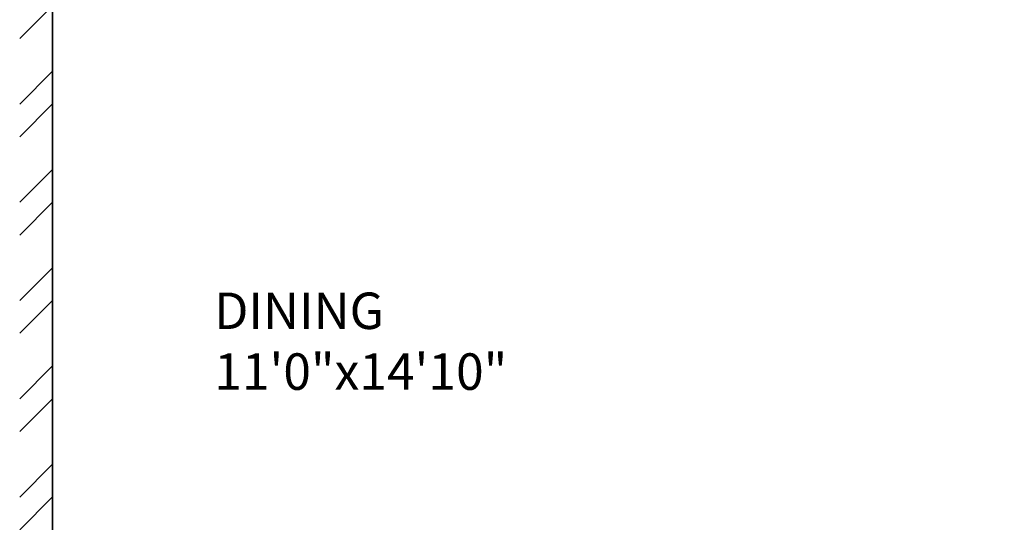
# Model space of a CAD drawing. Units: inches. Extents: x 1962 to 2771, y 1245 to 2660.
# Tile 12 of 114: x 2371 to 2506, y 1762 to 1831. Entities that reach past the tile are written whole.
import ezdxf

# ---------------------------------------------------------------- set-up
doc = ezdxf.new("R2010")
doc.units = ezdxf.units.IN
for name, color, linetype, lineweight in [('A-AREA-IDEN', 7, 'Continuous', 18), ('A-WALL', 7, 'Continuous', 35), ('A-WALL-PATT', 252, 'Continuous', 13)]:
    doc.layers.add(name, color=color, linetype=linetype, lineweight=lineweight)
doc.styles.get("Standard").update_dxf_attribs({"font": 'arial.ttf'})

msp = doc.modelspace()

# ---------------------------------------------------------------- hatches: boundary and pattern name
at = {"layer": 'A-WALL-PATT'}
h = msp.add_hatch(dxfattribs=at)
h.set_pattern_fill('ANSI32', color=256)
h.paths.add_polyline_path([(2090.8074, 2467.3437), (2141.6481, 2467.3437), (2141.6481, 2469.5937), (2141.6481, 2471.8437), (2086.3074, 2471.8437), (2086.3074, 2422.5333), (2090.8074, 2422.5333)])
h.paths.add_polyline_path([(2282.7664, 2471.8437), (2204.8982, 2471.8437), (2204.8982, 2467.3437), (2234.8074, 2467.3437), (2234.8074, 2311.3437), (2228.7492, 2311.3437), (2228.7492, 2306.8437), (2234.8074, 2306.8437), (2331.9227, 2306.8437), (2331.9227, 2309.0937), (2331.9227, 2311.3437), (2239.3074, 2311.3437), (2239.3074, 2467.3437), (2282.7664, 2467.3437), (2282.7664, 2469.5937)])
h.paths.add_polyline_path([(2471.4531, 2519.8437), (2552.011, 2519.8437), (2564.3996, 2519.8437), (2564.3996, 2511.1389), (2568.8996, 2511.1389), (2568.8996, 2524.3437), (2466.9531, 2524.3437), (2466.9531, 2471.8437), (2450.0749, 2471.8437), (2446.4672, 2471.8437), (2446.4672, 2467.3437), (2450.0749, 2467.3437), (2475.9988, 2467.3437), (2475.9988, 2469.5937), (2475.9988, 2471.8437), (2471.4531, 2471.8437)])
h.paths.add_polyline_path([(2575.2231, 2469.5937), (2575.2231, 2471.8437), (2568.8996, 2471.8437), (2568.8996, 2487.1389), (2564.3996, 2487.1389), (2564.3996, 2471.8437), (2556.511, 2471.8437), (2499.2904, 2471.8437), (2499.2904, 2467.3437), (2507.8074, 2467.3437), (2507.8074, 2311.3437), (2414.863, 2311.3437), (2414.863, 2306.8437), (2512.3074, 2306.8437), (2517.0114, 2306.8437), (2517.0114, 2309.0937), (2517.0114, 2311.3437), (2512.3074, 2311.3437), (2512.3074, 2467.3437), (2575.2231, 2467.3437)])
h.paths.add_polyline_path([(2660.8074, 2471.8437), (2600.9602, 2471.8437), (2600.9602, 2467.3437), (2656.3074, 2467.3437), (2656.3074, 2432.5704), (2660.8074, 2432.5704)])
h.paths.add_polyline_path([(2660.8074, 2372.5704), (2656.3074, 2372.5704), (2656.3074, 2311.3437), (2600.276, 2311.3437), (2600.276, 2309.0937), (2600.276, 2306.8437), (2656.3074, 2306.8437), (2656.3074, 2296.2593), (2660.8074, 2296.2593)])
h.paths.add_polyline_path([(2572.3074, 2306.8437), (2577.1385, 2306.8437), (2577.1385, 2311.3437), (2551.082, 2311.3437), (2551.082, 2306.8437), (2567.8074, 2306.8437), (2567.8074, 2258.8437), (2540.0574, 2258.8437), (2540.0574, 2256.5937), (2540.0574, 2254.3437), (2567.8074, 2254.3437), (2656.3074, 2254.3437), (2656.3074, 2236.9085), (2660.8074, 2236.9085), (2660.8074, 2272.2593), (2656.3074, 2272.2593), (2656.3074, 2258.8437), (2572.3074, 2258.8437)])
h.paths.add_polyline_path([(2512.3074, 2254.3437), (2518.8716, 2254.3437), (2518.8716, 2256.5937), (2518.8716, 2258.8437), (2507.8074, 2258.8437), (2507.8074, 2177.8437), (2567.8074, 2177.8437), (2567.8074, 2172.9628), (2572.3074, 2172.9628), (2572.3074, 2177.8437), (2656.3074, 2177.8437), (2656.3074, 2166.4846), (2660.8074, 2166.4846), (2660.8074, 2200.9085), (2656.3074, 2200.9085), (2656.3074, 2182.3437), (2512.3074, 2182.3437)])
h.paths.add_polyline_path([(2656.3074, 2129.8437), (2572.3074, 2129.8437), (2572.3074, 2150.3044), (2570.0574, 2150.3044), (2567.8074, 2150.3044), (2567.8074, 2129.8437), (2507.8074, 2129.8437), (2507.8074, 2116.3027), (2510.0574, 2116.3027), (2512.3074, 2116.3027), (2512.3074, 2125.3437), (2567.8074, 2125.3437), (2572.3074, 2125.3437), (2656.3074, 2125.3437)])
h.paths.add_polyline_path([(2090.8074, 2362.5333), (2086.3074, 2362.5333), (2086.3074, 2298.6242), (2090.8074, 2298.6242), (2090.8074, 2306.8437), (2174.8074, 2306.8437), (2174.8074, 2286.4178), (2179.3074, 2286.4178), (2179.3074, 2306.8437), (2192.8641, 2306.8437), (2192.8641, 2309.0937), (2192.8641, 2311.3437), (2090.8074, 2311.3437)])
h.paths.add_polyline_path([(2209.156, 2258.8437), (2179.3074, 2258.8437), (2179.3074, 2263.2236), (2177.0574, 2263.2236), (2174.8074, 2263.2236), (2174.8074, 2258.8437), (2090.8074, 2258.8437), (2090.8074, 2274.6242), (2086.3074, 2274.6242), (2086.3074, 2238.2967), (2088.5574, 2238.2967), (2090.8074, 2238.2967), (2090.8074, 2254.3437), (2209.156, 2254.3437)])
h.paths.add_polyline_path([(2090.8074, 2177.8437), (2234.8074, 2177.8437), (2234.8074, 2173.1428), (2239.3074, 2173.1428), (2239.3074, 2258.8437), (2230.8442, 2258.8437), (2230.8442, 2256.5937), (2230.8442, 2254.3437), (2234.8074, 2254.3437), (2234.8074, 2182.3437), (2090.8074, 2182.3437), (2090.8074, 2202.2967), (2086.3074, 2202.2967), (2086.3074, 2140.0389), (2090.8074, 2140.0389)])
h.paths.add_polyline_path([(2090.8074, 2080.0389), (2086.3074, 2080.0389), (2086.3074, 2033.8437), (2090.8074, 2033.8437)], flags=17)
h.paths.add_polyline_path([(2244.9405, 2033.8437), (2239.3074, 2033.8437), (2239.3074, 2142.0665), (2237.2592, 2142.0665), (2234.8074, 2142.0665), (2234.8074, 2033.8437), (2090.8074, 2033.8437), (2076.5204, 2033.8437), (2072.0204, 2033.8437), (2072.0204, 2000.4493), (2076.5204, 2000.4493), (2076.5204, 2029.3437), (2090.8074, 2029.3437), (2244.9405, 2029.3437), (2244.9405, 2031.5937)])
h.paths.add_polyline_path([(2234.8074, 1933.3437), (2076.5204, 1933.3437), (2076.5204, 1952.4493), (2074.2704, 1952.4493), (2072.0204, 1952.4493), (2072.0204, 1933.3437), (2072.0204, 1928.8437), (2234.8074, 1928.8437)])
h.paths.add_polyline_path([(2090.8074, 1928.8437), (2086.3074, 1928.8437), (2086.3074, 1906.5013), (2090.8074, 1906.5013)])
h.paths.add_polyline_path([(2090.8074, 1846.5013), (2086.3074, 1846.5013), (2086.3074, 1769.9917), (2088.5574, 1769.9917), (2090.8074, 1769.9917), (2090.8074, 1780.3437), (2234.8074, 1780.3437), (2234.8074, 1708.3437), (2230.3764, 1708.3437), (2230.3764, 1703.8437), (2239.3074, 1703.8437), (2239.3074, 1792.6669), (2237.0574, 1792.6669), (2234.8074, 1792.6669), (2234.8074, 1784.8437), (2090.8074, 1784.8437)])
h.paths.add_polyline_path([(2239.3074, 1928.8437), (2244.9405, 1928.8437), (2244.9405, 1931.0937), (2244.9405, 1933.3437), (2234.8074, 1933.3437), (2234.8074, 1928.8437), (2234.8074, 1825.5949), (2239.3074, 1825.5949)])
h.paths.add_polyline_path([(2148.0425, 1649.0937), (2148.0425, 1651.3437), (2090.8074, 1651.3437), (2090.8074, 1646.8437), (2148.0425, 1646.8437)], flags=0)
h.paths.add_polyline_path([(2207.5601, 1708.3437), (2090.8074, 1708.3437), (2090.8074, 1703.8437), (2174.8074, 1703.8437), (2174.8074, 1651.3437), (2170.4457, 1651.3437), (2170.4457, 1646.8437), (2195.9924, 1646.8437), (2195.9924, 1649.0937), (2195.9924, 1651.3437), (2179.3074, 1651.3437), (2179.3074, 1703.8437), (2207.5601, 1703.8437), (2207.5601, 1706.0937)])
h.paths.add_polyline_path([(2090.8074, 1733.9917), (2086.3074, 1733.9917), (2086.3074, 1696.1032), (2088.5574, 1696.1032), (2090.8074, 1696.1032)])
h.paths.add_polyline_path([(2090.8074, 1672.1032), (2086.3074, 1672.1032), (2086.3074, 1600.3335), (2090.8074, 1600.3335)])
h.paths.add_polyline_path([(2090.8074, 1540.3335), (2086.3074, 1540.3335), (2086.3074, 1486.3437), (2139.6766, 1486.3437), (2139.6766, 1490.8437), (2090.8074, 1490.8437)])
h.paths.add_polyline_path([(2302.3876, 1490.8437), (2239.3074, 1490.8437), (2239.3074, 1646.8437), (2335.9994, 1646.8437), (2335.9994, 1651.3437), (2229.884, 1651.3437), (2229.884, 1646.8437), (2234.8074, 1646.8437), (2234.8074, 1490.8437), (2202.7103, 1490.8437), (2202.7103, 1488.5937), (2202.7103, 1486.3437), (2275.0699, 1486.3437), (2275.0699, 1475.772), (2279.5699, 1475.772), (2279.5699, 1486.3437), (2302.3876, 1486.3437)])
h.paths.add_polyline_path([(2279.5699, 1451.772), (2275.0699, 1451.772), (2275.0699, 1438.3437), (2174.8074, 1438.3437), (2174.8074, 1486.3437), (2179.7922, 1486.3437), (2179.7922, 1490.8437), (2163.3585, 1490.8437), (2163.3585, 1488.5937), (2163.3585, 1486.3437), (2170.3074, 1486.3437), (2170.3074, 1433.8437), (2279.5699, 1433.8437)])
h.paths.add_polyline_path([(2427.2363, 1490.8437), (2375.8074, 1490.8437), (2375.8074, 1646.8437), (2381.6401, 1646.8437), (2381.6401, 1651.3437), (2365.887, 1651.3437), (2365.887, 1649.0937), (2365.887, 1646.8437), (2371.3074, 1646.8437), (2371.3074, 1490.8437), (2327.5627, 1490.8437), (2327.5627, 1488.5937), (2327.5627, 1486.3437), (2371.3074, 1486.3437), (2371.3074, 1433.8437), (2375.8074, 1433.8437), (2375.8074, 1486.3437), (2427.2363, 1486.3437)])
h.paths.add_polyline_path([(2512.3074, 1646.8437), (2519.4351, 1646.8437), (2519.4351, 1649.0937), (2519.4351, 1651.3437), (2507.8074, 1651.3437), (2416.0063, 1651.3437), (2416.0063, 1649.0937), (2416.0063, 1646.8437), (2507.8074, 1646.8437), (2507.8074, 1490.8437), (2497.0532, 1490.8437), (2497.0532, 1488.5937), (2497.0532, 1486.3437), (2574.9344, 1486.3437), (2574.9344, 1476.0181), (2579.4344, 1476.0181), (2579.4344, 1486.3437), (2584.4872, 1486.3437), (2584.3074, 1490.8437), (2512.3074, 1490.8437)])
h.paths.add_polyline_path([(2470.5091, 1486.3437), (2473.9767, 1486.3437), (2473.9767, 1490.8437), (2449.6605, 1490.8437), (2449.6605, 1488.5937), (2449.6605, 1486.3437), (2466.0091, 1486.3437), (2466.0091, 1433.8437), (2470.5091, 1433.8437), (2579.4344, 1433.8437), (2579.4344, 1452.0181), (2574.9344, 1452.0181), (2574.9344, 1438.3437), (2554.5091, 1438.3437), (2470.5091, 1438.3437)])
h.paths.add_polyline_path([(2656.3074, 1490.8437), (2611.86, 1490.8437), (2611.86, 1486.3437), (2656.3074, 1486.3437)])
h.paths.add_polyline_path([(2660.8074, 1532.7007), (2658.5574, 1532.7007), (2656.3074, 1532.7007), (2656.3074, 1486.3437), (2660.8074, 1486.3437)])
h.paths.add_polyline_path([(2660.8074, 1664.9663), (2656.3074, 1664.9663), (2656.3074, 1651.3437), (2602.2313, 1651.3437), (2602.2313, 1646.8437), (2656.3074, 1646.8437), (2656.3074, 1592.7007), (2660.8074, 1592.7007)])
h.paths.add_polyline_path([(2660.8074, 1724.5221), (2656.3074, 1724.5221), (2656.3074, 1703.8437), (2542.4725, 1703.8437), (2542.4725, 1699.3437), (2567.8074, 1699.3437), (2567.8074, 1651.3437), (2552.7766, 1651.3437), (2552.7766, 1649.0937), (2552.7766, 1646.8437), (2577.2878, 1646.8437), (2577.2878, 1649.0937), (2577.2878, 1651.3437), (2572.3074, 1651.3437), (2572.3074, 1699.3437), (2656.3074, 1699.3437), (2656.3074, 1688.9663), (2660.8074, 1688.9663)])
h.paths.add_polyline_path([(2660.8074, 1880.6524), (2656.3074, 1880.6524), (2656.3074, 1832.8437), (2512.3074, 1832.8437), (2512.3074, 1837.8959), (2507.8074, 1837.8959), (2507.8074, 1828.3437), (2567.8074, 1828.3437), (2567.8074, 1804.3437), (2572.3074, 1804.3437), (2572.3074, 1828.3437), (2656.3074, 1828.3437), (2656.3074, 1818.6778), (2660.8074, 1818.6778)])
h.paths.add_polyline_path([(2660.8074, 1794.6778), (2656.3074, 1794.6778), (2656.3074, 1780.3437), (2572.3074, 1780.3437), (2572.3074, 1783.0303), (2570.0574, 1783.0303), (2567.8074, 1783.0303), (2567.8074, 1780.3437), (2507.8074, 1780.3437), (2507.8074, 1699.3437), (2517.8858, 1699.3437), (2517.8858, 1701.5937), (2517.8858, 1703.8437), (2512.3074, 1703.8437), (2512.3074, 1775.8437), (2656.3074, 1775.8437), (2656.3074, 1760.5221), (2660.8074, 1760.5221)])
h.paths.add_polyline_path([(2660.8074, 1981.3437), (2660.8074, 2020.2808), (2658.5574, 2020.2808), (2656.3074, 2020.2808), (2656.3074, 1981.3437), (2512.3074, 1981.3437), (2512.3074, 2086.6996), (2507.8074, 2086.6996), (2507.8074, 1981.3437), (2375.8074, 1981.3437), (2375.8074, 1986.8505), (2373.5574, 1986.8505), (2371.3074, 1986.8505), (2371.3074, 1973.2607), (2375.8074, 1973.2607), (2375.8074, 1976.8437), (2507.8074, 1976.8437), (2507.8074, 1865.4281), (2510.0574, 1865.4281), (2512.3074, 1865.4281), (2512.3074, 1976.8437), (2660.8074, 1976.8437)])
h.paths.add_polyline_path([(2375.8074, 1940.297), (2373.5574, 1940.297), (2371.3074, 1940.297), (2371.3074, 1933.3437), (2278.4434, 1933.3437), (2278.4434, 1928.8437), (2371.3074, 1928.8437), (2371.3074, 1651.3437), (2375.8074, 1651.3437)])
h.paths.add_polyline_path([(2660.8074, 1976.8437), (2656.3074, 1976.8437), (2656.3074, 1940.6524), (2660.8074, 1940.6524)], flags=17)
h.paths.add_polyline_path([(2660.8074, 2142.4846), (2656.3074, 2142.4846), (2656.3074, 2080.2808), (2660.8074, 2080.2808)])
h.paths.add_polyline_path([(2381.4189, 2311.3437), (2375.8074, 2311.3437), (2375.8074, 2467.3437), (2424.7242, 2467.3437), (2424.7242, 2469.5937), (2424.7242, 2471.8437), (2375.8074, 2471.8437), (2375.8074, 2524.3437), (2371.3074, 2524.3437), (2371.3074, 2471.8437), (2307.2097, 2471.8437), (2307.2097, 2467.3437), (2371.3074, 2467.3437), (2371.3074, 2311.3437), (2366.8901, 2311.3437), (2366.8901, 2306.8437), (2371.3074, 2306.8437), (2371.3074, 2033.8437), (2279.6589, 2033.8437), (2279.6589, 2029.3437), (2371.3074, 2029.3437), (2371.3074, 2014.2598), (2375.8074, 2014.2598), (2375.8074, 2306.8437), (2381.4189, 2306.8437)])
h.paths.add_polyline_path([(2263.3074, 2524.3437), (2170.3074, 2524.3437), (2170.3074, 2519.8437), (2170.3074, 2471.8437), (2165.0312, 2471.8437), (2165.0312, 2467.3437), (2179.6721, 2467.3437), (2179.6721, 2469.5161), (2179.6721, 2471.8437), (2174.8074, 2471.8437), (2174.8074, 2519.8437), (2258.8074, 2519.8437), (2258.8074, 2511.6436), (2263.3074, 2511.6436)])
h.paths.add_polyline_path([(2245.0232, 1361.4123), (2492.9468, 1361.4123), (2492.9468, 1398.505), (2245.0232, 1398.505)], flags=9)
h.paths.add_polyline_path([(2388.1434, 2086.6936), (2425.0704, 2086.6936), (2425.0704, 2105.3509), (2388.1434, 2105.3509)], flags=9)
h.paths.add_polyline_path([(2404.922, 2242.6744), (2445.7337, 2242.6744), (2445.7337, 2261.3318), (2404.922, 2261.3318)], flags=9)
h.paths.add_polyline_path([(2269.4107, 2156.7935), (2306.3378, 2156.7935), (2306.3378, 2175.4508), (2269.4107, 2175.4508)], flags=9)
h.paths.add_polyline_path([(2269.3277, 2233.4343), (2306.2547, 2233.4343), (2306.2547, 2252.0917), (2269.3277, 2252.0917)], flags=9)
h.paths.add_polyline_path([(2431.6052, 2320.6922), (2470.4456, 2320.6922), (2470.4456, 2339.3495), (2431.6052, 2339.3495)], flags=25)
h.paths.add_polyline_path([(2249.6902, 2315.7608), (2288.5306, 2315.7608), (2288.5306, 2334.4182), (2249.6902, 2334.4182)], flags=25)
h.paths.add_polyline_path([(2096.9301, 2314.3181), (2135.7704, 2314.3181), (2135.7704, 2332.9755), (2096.9301, 2332.9755)], flags=25)
h.paths.add_polyline_path([(2134.3475, 2285.7089), (2161.4655, 2285.7089), (2161.4655, 2304.3662), (2134.3475, 2304.3662)], flags=9)
h.paths.add_polyline_path([(2126.5155, 2209.4076), (2159.9227, 2209.4076), (2159.9227, 2228.065), (2126.5155, 2228.065)], flags=25)
h.paths.add_polyline_path([(2110.5753, 2141.5299), (2149.4157, 2141.5299), (2149.4157, 2160.1872), (2110.5753, 2160.1872)], flags=25)
h.paths.add_polyline_path([(2249.8618, 1968.3317), (2286.3966, 1968.3317), (2286.3966, 1986.989), (2249.8618, 1986.989)], flags=9)
h.paths.add_polyline_path([(2395.9507, 1777.0051), (2436.7624, 1777.0051), (2436.7624, 1795.6625), (2395.9507, 1795.6625)], flags=9)
h.paths.add_polyline_path([(2398.5259, 1888.5651), (2435.0062, 1888.5651), (2435.0062, 1907.2224), (2398.5259, 1907.2224)], flags=25)
h.paths.add_polyline_path([(2259.3506, 1728.3559), (2296.2776, 1728.3559), (2296.2776, 1747.0132), (2259.3506, 1747.0132)], flags=9)
h.paths.add_polyline_path([(2271.3698, 1845.268), (2308.2968, 1845.268), (2308.2968, 1863.9253), (2271.3698, 1863.9253)], flags=9)
h.paths.add_polyline_path([(2120.9355, 1786.3027), (2159.7759, 1786.3027), (2159.7759, 1804.9601), (2120.9355, 1804.9601)], flags=25)
h.paths.add_polyline_path([(2121.3164, 1732.1043), (2154.7236, 1732.1043), (2154.7236, 1750.7616), (2121.3164, 1750.7616)], flags=25)
h.paths.add_polyline_path([(2118.3706, 1678.8997), (2147.5282, 1678.8997), (2147.5282, 1697.557), (2118.3706, 1697.557)], flags=25)
h.paths.add_polyline_path([(2385.9227, 1493.557), (2424.763, 1493.557), (2424.763, 1512.2143), (2385.9227, 1512.2143)], flags=25)
h.paths.add_polyline_path([(2248.7058, 1500.0256), (2287.5462, 1500.0256), (2287.5462, 1518.6829), (2248.7058, 1518.6829)], flags=25)
h.paths.add_polyline_path([(2104.1669, 1617.3771), (2143.0073, 1617.3771), (2143.0073, 1636.0344), (2104.1669, 1636.0344)], flags=9)
h.paths.add_polyline_path([(2096.0714, 1447.8824), (2137.3845, 1447.8824), (2137.3845, 1458.1859), (2096.0714, 1458.1859)], flags=9)
h.paths.add_polyline_path([(2180.6114, 1440.325), (2209.7689, 1440.325), (2209.7689, 1458.9823), (2180.6114, 1458.9823)], flags=25)
h.paths.add_polyline_path([(2316.1698, 1447.9637), (2357.4829, 1447.9637), (2357.4829, 1458.2673), (2316.1698, 1458.2673)], flags=9)
h.paths.add_polyline_path([(2397.6187, 1447.9637), (2438.9318, 1447.9637), (2438.9318, 1458.2673), (2397.6187, 1458.2673)], flags=9)
h.paths.add_polyline_path([(2473.0778, 1439.5953), (2502.2354, 1439.5953), (2502.2354, 1458.2527), (2473.0778, 1458.2527)], flags=25)
h.paths.add_polyline_path([(2589.7027, 1447.8819), (2631.0158, 1447.8819), (2631.0158, 1458.1855), (2589.7027, 1458.1855)], flags=9)
h.paths.add_polyline_path([(2522.4009, 1497.5285), (2561.2413, 1497.5285), (2561.2413, 1516.1859), (2522.4009, 1516.1859)], flags=25)
h.paths.add_polyline_path([(2579.6565, 1671.3482), (2608.8141, 1671.3482), (2608.8141, 1690.0056), (2579.6565, 1690.0056)], flags=25)
h.paths.add_polyline_path([(2544.7038, 1725.5064), (2578.1111, 1725.5064), (2578.1111, 1744.1637), (2544.7038, 1744.1637)], flags=25)
h.paths.add_polyline_path([(2578.1191, 1807.472), (2607.2766, 1807.472), (2607.2766, 1826.1293), (2578.1191, 1826.1293)], flags=25)
h.paths.add_polyline_path([(2595.0614, 1835.1839), (2633.9018, 1835.1839), (2633.9018, 1853.8413), (2595.0614, 1853.8413)], flags=25)
h.paths.add_polyline_path([(2567.0097, 2097.7035), (2605.8501, 2097.7035), (2605.8501, 2116.3609), (2567.0097, 2116.3609)], flags=9)
h.paths.add_polyline_path([(2586.644, 2134.6454), (2615.8015, 2134.6454), (2615.8015, 2153.3027), (2586.644, 2153.3027)], flags=9)
h.paths.add_polyline_path([(2544.6185, 2212.6783), (2578.0258, 2212.6783), (2578.0258, 2231.3356), (2544.6185, 2231.3356)], flags=25)
h.paths.add_polyline_path([(2577.0273, 2256.9023), (2606.1849, 2256.9023), (2606.1849, 2275.5597), (2577.0273, 2275.5597)], flags=24)
h.paths.add_polyline_path([(2605.2683, 2315.2821), (2644.1087, 2315.2821), (2644.1087, 2333.9395), (2605.2683, 2333.9395)], flags=25)
h.paths.add_polyline_path([(2583.1244, 2496.1815), (2624.4375, 2496.1815), (2624.4375, 2506.4851), (2583.1244, 2506.4851)], flags=9)
h.paths.add_polyline_path([(2474.761, 2497.0823), (2503.9185, 2497.0823), (2503.9185, 2515.7397), (2474.761, 2515.7397)], flags=25)
h.paths.add_polyline_path([(2387.5787, 2494.2563), (2428.902, 2494.2563), (2428.902, 2504.5598), (2387.5787, 2504.5598)], flags=9)
h.paths.add_polyline_path([(2300.1657, 2500.1564), (2341.4788, 2500.1564), (2341.4788, 2510.46), (2300.1657, 2510.46)], flags=25)
h.paths.add_polyline_path([(2176.8589, 2497.5843), (2206.0165, 2497.5843), (2206.0165, 2516.2416), (2176.8589, 2516.2416)], flags=25)
h.paths.add_polyline_path([(2097.4668, 2494.9762), (2138.7799, 2494.9762), (2138.7799, 2505.2798), (2097.4668, 2505.2798)], flags=9)

# ---------------------------------------------------------------- linework, layer by layer
at = {"layer": 'A-WALL'}
msp.add_line((2375.8074, 1941.894), (2375.8074, 1651.3437), dxfattribs=at)

# ---------------------------------------------------------------- texts
at = {"layer": 'A-AREA-IDEN', "insert": (2397.9612, 1793.1744), "char_height": 5, "attachment_point": 1}
msp.add_mtext_dynamic_manual_height_columns('DINING\\P11\'0"x14\'10"', width=163.504372, gutter_width=12.5, heights=[0], dxfattribs=at)

doc.saveas('drawing.dxf')
